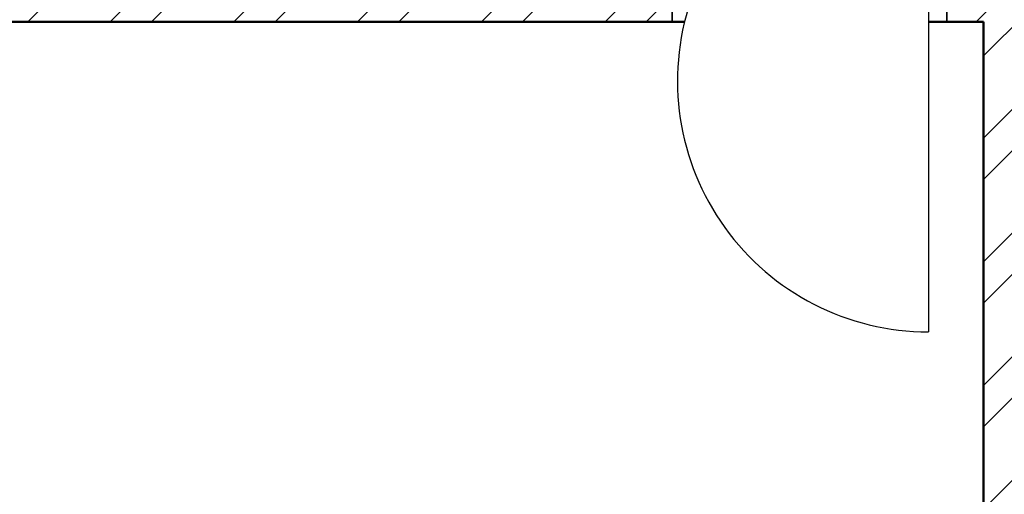
# Model space of a CAD drawing. Units: inches. Extents: x 963 to 2075, y 289 to 2657.
# Tile 27 of 98: x 1403 to 1511, y 1820 to 1872. Entities that reach past the tile are written whole.
import ezdxf

# ---------------------------------------------------------------- set-up
doc = ezdxf.new("R2010")
doc.units = ezdxf.units.IN
for name, color, linetype, lineweight in [('A-DOOR', 4, 'Continuous', 25), ('A-WALL', 7, 'Continuous', 50), ('A-WALL-PATT', 8, 'Continuous', 13)]:
    doc.layers.add(name, color=color, linetype=linetype, lineweight=lineweight)

# ---------------------------------------------------------------- blocks, each defined once
blk = doc.blocks.new('DOOR-5')
for p, q in [((0, 38.25), (0, 33.75)), ((29.91, 38.25), (29.91, 33.75)), ((0, 33.75), (0, 36)), ((0, 36), (2, 36)), ((29.91, 36), (27.91, 36)), ((27.91, 36), (27.91, 0)), ((29.91, 33.75), (29.91, 36))]:
    blk.add_line(p, q)
blk.add_arc((27.91, 27.32), 27.32, 161.4794, 270)

msp = doc.modelspace()

# ---------------------------------------------------------------- hatches: boundary and pattern name
at = {"layer": 'A-WALL-PATT'}
h = msp.add_hatch(dxfattribs=at)
h.set_pattern_fill('ANSI32', color=256)
h.paths.add_polyline_path([(1473.61, 2163.07), (1473.61, 2165.32), (1376.42, 2165.32), (1376.42, 2227.98), (1371.92, 2227.98), (1371.92, 2214.82), (1368.41, 2214.82), (1368.41, 2210.32), (1371.92, 2210.32), (1371.92, 2160.82), (1395.92, 2160.82), (1395.92, 2090.32), (1217.34, 2090.32), (1217.34, 2085.82), (1395.92, 2085.82), (1458.92, 2085.82), (1458.92, 2108.32), (1454.42, 2108.32), (1454.42, 2090.32), (1400.42, 2090.32), (1400.42, 2160.82), (1473.61, 2160.82)])
h.paths.add_polyline_path([(1649.42, 2210.32), (1653.23, 2210.32), (1653.23, 2214.82), (1649.42, 2214.82), (1649.42, 2227.98), (1644.92, 2227.98), (1644.92, 2165.32), (1550.1, 2165.32), (1550.1, 2160.82), (1620.92, 2160.82), (1620.92, 2112.82), (1555.45, 2112.82), (1555.45, 2108.32), (1584.33, 2108.32), (1584.33, 2084.92), (1588.83, 2084.92), (1588.83, 2108.32), (1625.42, 2108.32), (1667.95, 2108.32), (1667.95, 2022.67), (1588.83, 2022.67), (1588.83, 2047.41), (1584.33, 2047.41), (1584.33, 1996), (1588.83, 1996), (1588.83, 2018.32), (1667.95, 2018.17), (1667.95, 1928.32), (1625.42, 1928.32), (1625.42, 1923.82), (1672.45, 1923.82), (1672.45, 1928.32), (1672.45, 1946.66), (1785.45, 1946.66), (1785.45, 1951.16), (1743.03, 1951.16), (1743.03, 2017.92), (1841.42, 2017.92), (1841.42, 2014.77), (1845.92, 2014.77), (1845.92, 2017.92), (1905.92, 2017.92), (1905.92, 1987.51), (1910.42, 1987.51), (1910.42, 2022.42), (1910.42, 2068.52), (1905.92, 2068.52), (1905.92, 2022.42), (1845.92, 2022.42), (1845.92, 2025.85), (1843.67, 2025.85), (1841.42, 2025.85), (1841.42, 2022.42), (1743.03, 2022.42), (1743.03, 2084.03), (1768.45, 2084.03), (1785.45, 2084.03), (1785.45, 2088.53), (1672.45, 2088.53), (1672.45, 2112.82), (1667.95, 2112.82), (1625.42, 2112.82), (1625.42, 2160.82), (1649.42, 2160.82)])
h.paths.add_polyline_path([(1672.45, 2084.03), (1738.53, 2084.03), (1738.53, 1951.16), (1672.45, 1951.16)], flags=16)
h.paths.add_polyline_path([(1672.45, 2084.03), (1738.53, 2084.03), (1705.49, 2017.6)], flags=0)
h.paths.add_polyline_path([(1262.77, 2085.82), (1258.27, 2085.82), (1258.27, 2023.28), (1184.42, 2023.28), (1184.42, 2018.78), (1258.27, 2018.78), (1258.27, 1950.82), (1262.77, 1950.82)])
h.paths.add_polyline_path([(1312.27, 2085.82), (1307.77, 2085.82), (1307.77, 1950.82), (1312.27, 1950.82)])
h.paths.add_polyline_path([(1458.92, 1950.82), (1395.92, 1950.82), (1216.57, 1950.82), (1216.57, 1946.32), (1346.42, 1946.32), (1395.92, 1946.32), (1395.92, 1875.82), (1371.92, 1875.82), (1371.92, 1826.32), (1368.93, 1826.32), (1368.93, 1821.82), (1371.92, 1821.82), (1371.92, 1813.62), (1376.42, 1813.62), (1376.42, 1871.32), (1474.5, 1871.32), (1474.5, 1873.57), (1474.5, 1875.82), (1400.42, 1875.82), (1400.42, 1946.32), (1454.42, 1946.32), (1454.42, 1928.32), (1458.92, 1928.32)])
h.paths.add_polyline_path([(1184.42, 2120.78), (1167.92, 2120.78), (1167.92, 2134.81), (1165.67, 2134.81), (1163.42, 2134.81), (1163.42, 2120.78), (1119.92, 2120.78), (1119.92, 2098.1), (1124.42, 2098.1), (1124.42, 2116.28), (1167.92, 2116.28), (1179.92, 2116.28), (1179.92, 2045.92), (1184.42, 2045.92), (1184.42, 2090.32), (1184.42, 2116.28)])
h.paths.add_polyline_path([(1124.42, 2018.78), (1179.92, 2018.78), (1179.92, 2016.29), (1184.42, 2016.29), (1184.42, 2023.28), (1184.42, 2026.59), (1182.17, 2026.59), (1179.92, 2026.59), (1179.92, 2023.28), (1124.42, 2023.28), (1124.42, 2074.1), (1119.92, 2074.1), (1119.92, 2018.78), (1119.92, 1979.63), (1124.42, 1979.63)])
h.paths.add_polyline_path([(1184.42, 1925.78), (1184.42, 1946.32), (1184.42, 1996.07), (1182.17, 1996.07), (1179.92, 1996.07), (1179.92, 1925.78), (1124.42, 1925.78), (1124.42, 1955.63), (1119.92, 1955.5), (1119.92, 1921.28), (1158.92, 1921.28), (1158.92, 1909.98), (1163.42, 1909.98), (1163.42, 1921.28), (1184.42, 1921.28)])
h.paths.add_polyline_path([(1341.45, 1826.32), (1163.42, 1826.32), (1163.42, 1849.98), (1158.92, 1849.98), (1158.92, 1821.82), (1158.92, 1804.03), (1163.42, 1804.03), (1163.42, 1821.82), (1341.45, 1821.82)])
h.paths.add_polyline_path([(1222.98, 1713.82), (1163.42, 1713.82), (1163.42, 1744.03), (1161.17, 1744.03), (1158.92, 1744.03), (1158.92, 1713.82), (1119.92, 1713.82), (1119.92, 1694.65), (1124.42, 1694.65), (1124.42, 1709.32), (1158.92, 1709.32), (1222.98, 1709.32)])
h.paths.add_polyline_path([(1328.42, 1713.82), (1252.04, 1713.82), (1252.04, 1711.57), (1252.04, 1709.32), (1256.42, 1709.32), (1256.42, 1547.32), (1232.94, 1547.32), (1232.94, 1545.07), (1232.94, 1542.82), (1292.42, 1542.82), (1292.42, 1527.63), (1296.92, 1527.63), (1296.92, 1542.82), (1299.46, 1542.82), (1299.46, 1547.32), (1260.92, 1547.32), (1260.92, 1658.32), (1343.66, 1658.32), (1343.66, 1660.57), (1343.66, 1662.82), (1328.42, 1662.82), (1328.42, 1676.59), (1327.4, 1676.59), (1323.92, 1676.59), (1323.92, 1662.82), (1260.92, 1662.82), (1260.92, 1709.32), (1323.92, 1709.32), (1323.92, 1699.85), (1328.42, 1699.85)])
h.paths.add_polyline_path([(1649.42, 1875.82), (1625.42, 1875.82), (1625.42, 1928.32), (1620.92, 1928.32), (1588.83, 1928.32), (1588.83, 1950.59), (1584.33, 1950.59), (1584.33, 1928.32), (1555.45, 1928.32), (1555.45, 1923.82), (1620.92, 1923.82), (1620.92, 1875.82), (1548.95, 1875.82), (1548.95, 1873.57), (1548.95, 1871.32), (1644.92, 1871.32), (1644.92, 1813.62), (1649.42, 1813.62), (1649.42, 1821.82), (1652.04, 1821.82), (1652.04, 1824.07), (1652.04, 1826.32), (1649.42, 1826.32)])
h.paths.add_polyline_path([(1512.92, 1871.32), (1516.48, 1871.32), (1516.48, 1875.82), (1512.92, 1875.82), (1512.92, 1923.82), (1512.92, 1928.32), (1512.92, 1930.83), (1508.42, 1930.83), (1508.42, 1875.82), (1504.41, 1875.82), (1504.41, 1871.32), (1508.42, 1871.32), (1508.42, 1713.82), (1376.42, 1713.82), (1376.42, 1743.32), (1371.92, 1743.32), (1371.92, 1709.32), (1371.92, 1706.01), (1376.42, 1706.01), (1376.42, 1709.32), (1508.42, 1709.32), (1508.42, 1547.32), (1501.87, 1547.32), (1501.87, 1542.82), (1508.42, 1542.82), (1508.42, 1482.82), (1508.42, 1436.32), (1512.92, 1436.32), (1512.92, 1542.82), (1519.32, 1542.82), (1519.32, 1545.07), (1519.32, 1547.32), (1512.92, 1547.32), (1512.92, 1709.32), (1644.92, 1709.32), (1644.92, 1707.55), (1649.42, 1707.55), (1649.42, 1709.32), (1649.42, 1743.32), (1644.92, 1743.32), (1644.92, 1713.82), (1512.92, 1713.82)])
h.paths.add_polyline_path([(1129.88, 1545.07), (1129.88, 1547.32), (1124.42, 1547.32), (1095.92, 1547.32), (1095.92, 1614.82), (1124.42, 1614.82), (1124.42, 1619.32), (1095.92, 1619.32), (1091.42, 1619.32), (1091.42, 1542.82), (1095.92, 1542.82), (1119.92, 1542.82), (1129.88, 1542.82)])
h.paths.add_polyline_path([(1208.42, 1542.82), (1211.74, 1542.82), (1211.74, 1547.32), (1198.85, 1547.32), (1198.85, 1542.82), (1203.92, 1542.82), (1203.92, 1478.32), (1208.42, 1478.32), (1296.92, 1478.32), (1296.92, 1503.63), (1292.42, 1503.63), (1292.42, 1482.82), (1208.42, 1482.82)])
h.paths.add_polyline_path([(1430.42, 1542.82), (1435.7, 1542.82), (1435.7, 1545.07), (1435.7, 1547.32), (1422.66, 1547.32), (1422.66, 1545.07), (1422.66, 1542.82), (1425.92, 1542.82), (1425.92, 1482.86), (1341.92, 1482.86), (1341.92, 1502.73), (1337.42, 1502.73), (1337.42, 1478.36), (1425.92, 1478.36), (1425.92, 1440.82), (1425.92, 1436.32), (1430.42, 1436.32)])
h.paths.add_polyline_path([(1698.48, 2004.26), (1727.69, 2004.26), (1727.69, 2022.92), (1698.48, 2022.92)], flags=8)

# ---------------------------------------------------------------- linework, layer by layer
at = {"layer": 'A-WALL'}
for p, q in [((1475.86, 1871.32), (1376.42, 1871.32)), ((1508.42, 1871.32), (1502.41, 1871.32)), ((1508.42, 1871.32), (1508.42, 1713.82))]:
    msp.add_line(p, q, dxfattribs=at)

# ---------------------------------------------------------------- block references
at = {"layer": 'A-DOOR'}
msp.add_blockref('DOOR-5', (1474.5, 1837.57), dxfattribs=at)

doc.saveas('drawing.dxf')
